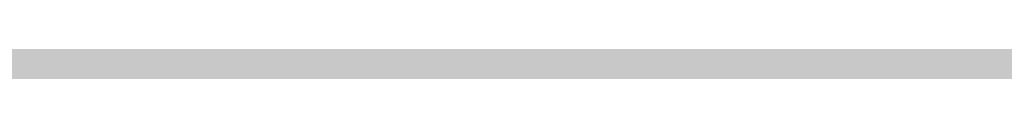
# Model space of a CAD drawing. Units: millimetres. Extents: x 0 to 2267, y 0 to 1823.
# Tile 205 of 256: x 1841.442 to 1842.748, y 1127.384 to 1127.404. Entities that reach past the tile are written whole.
import ezdxf

# ---------------------------------------------------------------- set-up
doc = ezdxf.new("R2010")
doc.units = ezdxf.units.MM
doc.header["$MEASUREMENT"] = 0
doc.layers.add('M-DIMS', color=2, linetype='Continuous', lineweight=25)
doc.layers.add('M-HATC', color=252, linetype='Continuous', lineweight=18)
doc.styles.get("Standard").update_dxf_attribs({"font": 'arial.ttf'})
doc.dimstyles.get("Standard").update_dxf_attribs({"dimtxt": 7, "dimasz": 4, "dimexe": 0.18, "dimexo": 0.0625, "dimgap": 0.09, "dimtad": 0, "dimdec": 0, "dimzin": 0, "dimdsep": 46, "dimtxsty": 'Standard', "dimcen": 0.09, "dimadec": 0, "dimazin": 0, "dimtfac": 1, "dimtdec": 0, "dimtofl": 0, "dimtmove": 0, "dimatfit": 3, "dimfxl": 1, "dimtolj": 1, "dimtzin": 0, "dimarcsym": 0})

# ---------------------------------------------------------------- blocks, each defined once
blk = doc.blocks.new('*D1')
at = {"layer": 'Defpoints', "color": 0, "transparency": 16777216}
for p in [(1593.4289, 1127.4171), (1843.4289, 1127.4171), (1843.4289, 955.6278)]:
    blk.add_point(p, dxfattribs=at)
at = {"layer": 'M-DIMS', "color": 0, "lineweight": -2, "transparency": 16777216}
for p, q in [((1593.4289, 1127.3546), (1593.4289, 955.4478)), ((1843.4289, 1127.3546), (1843.4289, 955.4478)), ((1597.4289, 955.6278), (1710.5582, 955.6278)), ((1839.4289, 955.6278), (1726.2996, 955.6278))]:
    blk.add_line(p, q, dxfattribs=at)
at = {"layer": 'M-DIMS', "color": 0, "transparency": 16777216}
for points in [[(1597.4289, 956.2944), (1597.4289, 954.9611), (1593.4289, 955.6278)], [(1839.4289, 956.2944), (1839.4289, 954.9611), (1843.4289, 955.6278)]]:
    blk.add_solid(points, dxfattribs=at)
at = {"layer": 'M-DIMS', "color": 0, "transparency": 16777216, "insert": (1718.4289, 955.6278), "char_height": 7, "attachment_point": 5}
blk.add_mtext('\\A1;250', dxfattribs=at)

msp = doc.modelspace()

# ---------------------------------------------------------------- hatches: boundary and pattern name
at = {"layer": 'M-HATC'}
h = msp.add_hatch(color=256, dxfattribs=at)
h.dxf.hatch_style = 1
h.paths.add_polyline_path([(2055.771, 1603.062), (1381.0868, 1603.062), (1381.0868, 1598.062), (2055.771, 1598.062)])
h.paths.add_polyline_path([(2055.771, 1598.062), (1381.0868, 1598.062), (1381.0868, 1593.062), (2055.771, 1593.062)])
h.paths.add_polyline_path([(2051.3074, 1536.7609), (1385.5504, 1536.7609), (1385.5504, 1526.7609), (1387.5504, 1526.7609), (1388.5366, 1525.0528), (1385.3319, 1521.2335), (1385.3319, 1521.2226), (2050.2542, 1522.7491), (2048.3212, 1525.0528), (2049.3074, 1526.7609), (2051.3074, 1526.7609)])
edge = h.paths.add_edge_path()
edge.add_arc((1847.5345, 1379.1492), 135, 222.603061, 222.890851, ccw=False)
edge.add_line((1748.1663, 1287.7656), (1683.0921, 1287.7656))
edge.add_arc((1583.7239, 1379.1492), 135, 317.109149, 317.396939, ccw=False)
edge.add_arc((1678.9686, 1290.6707), 5, 222.8909, 317.1091, ccw=False)
edge.add_arc((1774.2133, 1379.1492), 135, 222.603061, 222.890851, ccw=False)
edge.add_line((1674.8451, 1287.7656), (1609.7709, 1287.7656))
edge.add_arc((1510.4027, 1379.1492), 135, 317.109149, 317.396939, ccw=False)
edge.add_arc((1605.6474, 1290.6707), 5, 222.8909, 317.1091, ccw=False)
edge.add_arc((1700.8921, 1379.1492), 135, 222.603061, 222.890851, ccw=False)
edge.add_line((1601.5239, 1287.7656), (1536.4497, 1287.7656))
edge.add_arc((1437.0815, 1379.1492), 135, 317.109149, 317.396939, ccw=False)
edge.add_arc((1532.3262, 1290.6707), 5, 222.8909, 317.1091, ccw=False)
edge.add_arc((1627.5709, 1379.1492), 135, 222.603061, 222.890851, ccw=False)
edge.add_line((1528.2027, 1287.7656), (1505.9289, 1287.7656))
edge.add_spline(control_points=[(1505.9289, 1287.7656), (1504.2622, 1287.7656), (1504.2622, 1282.7656), (1505.9289, 1282.7656)], knot_values=[0, 0, 0, 0, 5, 5, 5, 5], degree=3, periodic=0)
edge.add_line((1505.9289, 1282.7656), (1930.9289, 1282.7656))
edge.add_spline(control_points=[(1930.9289, 1282.7656), (1932.5956, 1282.7656), (1932.5956, 1287.7656), (1930.9289, 1287.7656)], knot_values=[0, 0, 0, 0, 5, 5, 5, 5], degree=3, periodic=0)
edge.add_line((1930.9289, 1287.7656), (1903.0557, 1287.7656))
edge.add_arc((1803.6875, 1379.1492), 135, 317.109149, 317.396939, ccw=False)
edge.add_arc((1898.9322, 1290.6707), 5, 222.8909, 317.1091, ccw=False)
edge.add_arc((1994.1769, 1379.1492), 135, 222.603061, 222.890851, ccw=False)
edge.add_line((1894.8087, 1287.7656), (1829.7345, 1287.7656))
edge.add_arc((1730.3663, 1379.1492), 135, 317.109149, 317.396939, ccw=False)
edge.add_arc((1825.611, 1290.6707), 5, 222.8909, 317.1091, ccw=False)
edge.add_arc((1920.8557, 1379.1492), 135, 222.603061, 222.890851, ccw=False)
edge.add_line((1821.4875, 1287.7656), (1756.4133, 1287.7656))
edge.add_arc((1657.0451, 1379.1492), 135, 317.109149, 317.396939, ccw=False)
edge.add_arc((1752.2898, 1290.6707), 5, 222.8909, 317.1091, ccw=False)
edge = h.paths.add_edge_path()
edge.add_spline(control_points=[(1843.4289, 1227.2475), (1845.0956, 1227.2475), (1845.0956, 1232.2475), (1843.4289, 1232.2475)], knot_values=[0, 0, 0, 0, 5, 5, 5, 5], degree=3, periodic=0)
edge.add_line((1843.4289, 1232.2475), (1593.4289, 1232.2475))
edge.add_spline(control_points=[(1593.4289, 1232.2475), (1591.7622, 1232.2475), (1591.7622, 1227.2475), (1593.4289, 1227.2475)], knot_values=[0, 0, 0, 0, 5, 5, 5, 5], degree=3, periodic=0)
edge.add_line((1593.4289, 1227.2475), (1843.4289, 1227.2475))
h.paths.add_polyline_path([(1905.9289, 1127.4171), (1530.9289, 1127.4171, 0.414214), (1520.9289, 1117.4171), (1530.9289, 1117.4171), (1915.9289, 1117.4171, 0.414214)])
edge = h.paths.add_edge_path()
edge.add_arc((1397.0858, 1498.4078), 12.7299, 90.78215, 190.87871, ccw=False)
edge.add_line((1396.912, 1511.1365), (1428.0097, 1511.3488))
edge.add_line((1428.0097, 1511.3488), (1433.0097, 1511.3488))
edge.add_line((1433.0097, 1511.3488), (1434.439, 1511.3488))
edge.add_arc((1419.474, 1498.0804), 20, 41.561, 74.08211)
edge.add_line((1424.9592, 1517.3135), (1399.9351, 1517.2561))
edge.add_spline(control_points=[(1399.9307, 1517.2561), (1399.884, 1517.2131), (1399.8328, 1517.1689), (1399.7774, 1517.1236)], knot_values=[11.567499, 11.567499, 11.567499, 11.567499, 11.814249, 11.814249, 11.814249, 11.814249], degree=3, periodic=0)
edge.add_spline(control_points=[(1399.6328, 1517.0099), (1399.5831, 1516.9721), (1399.5307, 1516.9338), (1399.4759, 1516.8947)], knot_values=[11.167718, 11.167718, 11.167718, 11.167718, 11.365188, 11.365188, 11.365188, 11.365188], degree=3, periodic=0)
edge.add_spline(control_points=[(1399.3398, 1516.8001), (1399.1514, 1516.6719), (1398.9384, 1516.5377), (1398.704, 1516.3994)], knot_values=[10.376405, 10.376405, 10.376405, 10.376405, 11.00994, 11.00994, 11.00994, 11.00994], degree=3, periodic=0)
edge.add_spline(control_points=[(1398.6572, 1516.3719), (1398.5789, 1516.326), (1398.4983, 1516.2797), (1398.4155, 1516.2331)], knot_values=[10.125175, 10.125175, 10.125175, 10.125175, 10.334406, 10.334406, 10.334406, 10.334406], degree=3, periodic=0)
edge.add_spline(control_points=[(1398.2642, 1516.1487), (1398.196, 1516.1111), (1398.1263, 1516.0732), (1398.0555, 1516.0351)], knot_values=[9.832246, 9.832246, 9.832246, 9.832246, 9.999658, 9.999658, 9.999658, 9.999658], degree=3, periodic=0)
edge.add_spline(control_points=[(1397.9987, 1516.0048), (1397.7312, 1515.8621), (1397.446, 1515.7171), (1397.1466, 1515.5714)], knot_values=[9.161808, 9.161808, 9.161808, 9.161808, 9.787769, 9.787769, 9.787769, 9.787769], degree=3, periodic=0)
edge.add_spline(control_points=[(1397.1466, 1515.5714), (1396.8418, 1515.423), (1396.5222, 1515.274), (1396.1914, 1515.1262)], knot_values=[8.524455, 8.524455, 8.524455, 8.524455, 9.161808, 9.161808, 9.161808, 9.161808], degree=3, periodic=0)
edge.add_spline(control_points=[(1396.0777, 1515.0756), (1395.9854, 1515.0348), (1395.8922, 1514.994), (1395.7983, 1514.9534)], knot_values=[8.275193, 8.275193, 8.275193, 8.275193, 8.451726, 8.451726, 8.451726, 8.451726], degree=3, periodic=0)
edge.add_spline(control_points=[(1395.6018, 1514.8691), (1395.4997, 1514.8257), (1395.3968, 1514.7824), (1395.2932, 1514.7394)], knot_values=[7.962917, 7.962917, 7.962917, 7.962917, 8.152764, 8.152764, 8.152764, 8.152764], degree=3, periodic=0)
edge.add_spline(control_points=[(1395.2116, 1514.7057), (1394.8278, 1514.5475), (1394.4345, 1514.3929), (1394.0364, 1514.2442)], knot_values=[7.21254, 7.21254, 7.21254, 7.21254, 7.913148, 7.913148, 7.913148, 7.913148], degree=3, periodic=0)
edge.add_spline(control_points=[(1394.0364, 1514.2442), (1393.7076, 1514.1214), (1393.3754, 1514.0027), (1393.0427, 1513.8895)], knot_values=[6.633733, 6.633733, 6.633733, 6.633733, 7.21254, 7.21254, 7.21254, 7.21254], degree=3, periodic=0)
edge.add_spline(control_points=[(1392.8214, 1513.815), (1392.7198, 1513.7812), (1392.6181, 1513.7479), (1392.5166, 1513.7152)], knot_values=[6.328796, 6.328796, 6.328796, 6.328796, 6.505493, 6.505493, 6.505493, 6.505493], degree=3, periodic=0)
edge.add_spline(control_points=[(1392.5166, 1513.7152), (1392.3187, 1513.6515), (1392.1212, 1513.59), (1391.9244, 1513.531)], knot_values=[5.984605, 5.984605, 5.984605, 5.984605, 6.328796, 6.328796, 6.328796, 6.328796], degree=3, periodic=0)
edge.add_spline(control_points=[(1391.7915, 1513.4915), (1391.3122, 1513.3501), (1390.8384, 1513.2239), (1390.3784, 1513.1171)], knot_values=[5.066697, 5.066697, 5.066697, 5.066697, 5.907055, 5.907055, 5.907055, 5.907055], degree=3, periodic=0)
edge.add_spline(control_points=[(1390.3784, 1513.1171), (1390.1797, 1513.071), (1389.9836, 1513.0284), (1389.7907, 1512.9899)], knot_values=[4.70367, 4.70367, 4.70367, 4.70367, 5.066695, 5.066695, 5.066695, 5.066695], degree=3, periodic=0)
edge.add_spline(control_points=[(1389.422, 1512.9204), (1389.2459, 1512.8892), (1389.0729, 1512.8617), (1388.9036, 1512.8381)], knot_values=[4.130571, 4.130571, 4.130571, 4.130571, 4.469816, 4.469816, 4.469816, 4.469816], degree=3, periodic=0)
edge.add_spline(control_points=[(1388.9036, 1512.8381), (1388.591, 1512.7946), (1388.2911, 1512.7644), (1388.0071, 1512.7494)], knot_values=[3.504031, 3.504031, 3.504031, 3.504031, 4.130571, 4.130571, 4.130571, 4.130571], degree=3, periodic=0)
edge.add_spline(control_points=[(1387.9356, 1512.7459), (1387.8538, 1512.7423), (1387.7733, 1512.74), (1387.6944, 1512.739)], knot_values=[3.268866, 3.268866, 3.268866, 3.268866, 3.451164, 3.451164, 3.451164, 3.451164], degree=3, periodic=0)
edge.add_spline(control_points=[(1387.3351, 1512.7443), (1387.2076, 1512.7499), (1387.0847, 1512.7597), (1386.967, 1512.7739)], knot_values=[2.670686, 2.670686, 2.670686, 2.670686, 2.984, 2.984, 2.984, 2.984], degree=3, periodic=0)
edge.add_spline(control_points=[(1386.8327, 1512.7922), (1386.8209, 1512.7941), (1386.8092, 1512.7959), (1386.7975, 1512.7979)], knot_values=[2.516981, 2.516981, 2.516981, 2.516981, 2.549528, 2.549528, 2.549528, 2.549528], degree=3, periodic=0)
edge.add_spline(control_points=[(1386.4526, 1512.8735), (1386.4257, 1512.881), (1386.3993, 1512.889), (1386.3733, 1512.8972)], knot_values=[2.095869, 2.095869, 2.095869, 2.095869, 2.17941, 2.17941, 2.17941, 2.17941], degree=3, periodic=0)
edge.add_spline(control_points=[(1386.0691, 1513.0189), (1386.0634, 1513.0217), (1386.0577, 1513.0246), (1386.052, 1513.0275)], knot_values=[1.72453, 1.72453, 1.72453, 1.72453, 1.745933, 1.745933, 1.745933, 1.745933], degree=3, periodic=0)
edge.add_arc((1399.474, 1498.0804), 20, 131.82432, 180)
edge.add_arc((1630.3336, 1505.5484), 250.9708, 181.705176, 236.427975)
edge.add_arc((1605.3399, 1483.3044), 218.7822, 238.660829, 243.34961)
edge.add_arc((1647.0911, 1510.3592), 262.8986, 183.129836, 237.853442, ccw=False)
h.paths.add_polyline_path([(1406.5369, 1391.9644, 0.149382), (1491.5506, 1296.4418, -0.129517)], flags=17)
edge = h.paths.add_edge_path()
edge.add_arc((2037.3838, 1498.0804), 20, 0, 48.26587)
edge.add_spline(control_points=[(2050.6973, 1513.0052), (2050.6512, 1512.9847), (2050.6034, 1512.9655), (2050.5539, 1512.9477)], knot_values=[1.835652, 1.835652, 1.835652, 1.835652, 2.000781, 2.000781, 2.000781, 2.000781], degree=3, periodic=0)
edge.add_spline(control_points=[(2050.4616, 1512.9166), (2050.479, 1512.9221), (2050.4963, 1512.9277), (2050.5133, 1512.9335)], knot_values=[2.045477, 2.045477, 2.045477, 2.045477, 2.101389, 2.101389, 2.101389, 2.101389], degree=3, periodic=0)
edge.add_spline(control_points=[(2050.129, 1512.8342), (2050.1984, 1512.8473), (2050.2657, 1512.8623), (2050.3308, 1512.8792)], knot_values=[2.237629, 2.237629, 2.237629, 2.237629, 2.435841, 2.435841, 2.435841, 2.435841], degree=3, periodic=0)
edge.add_spline(control_points=[(2050.0946, 1512.8278), (2050.1061, 1512.8299), (2050.1176, 1512.832), (2050.129, 1512.8342)], knot_values=[2.435841, 2.435841, 2.435841, 2.435841, 2.468321, 2.468321, 2.468321, 2.468321], degree=3, periodic=0)
edge.add_spline(control_points=[(2049.7843, 1512.7851), (2049.8552, 1512.7922), (2049.9243, 1512.8008), (2049.9917, 1512.8109)], knot_values=[2.563852, 2.563852, 2.563852, 2.563852, 2.748541, 2.748541, 2.748541, 2.748541], degree=3, periodic=0)
edge.add_spline(control_points=[(2049.4052, 1512.7617), (2049.5364, 1512.7653), (2049.6629, 1512.773), (2049.7843, 1512.7851)], knot_values=[2.748541, 2.748541, 2.748541, 2.748541, 3.064882, 3.064882, 3.064882, 3.064882], degree=3, periodic=0)
edge.add_spline(control_points=[(2049.1698, 1512.7597), (2049.2336, 1512.7591), (2049.2965, 1512.7594), (2049.3584, 1512.7606)], knot_values=[3.102309, 3.102309, 3.102309, 3.102309, 3.2503, 3.2503, 3.2503, 3.2503], degree=3, periodic=0)
edge.add_spline(control_points=[(2048.8573, 1512.7691), (2048.9638, 1512.7638), (2049.068, 1512.7606), (2049.1698, 1512.7597)], knot_values=[3.2503, 3.2503, 3.2503, 3.2503, 3.486069, 3.486069, 3.486069, 3.486069], degree=3, periodic=0)
edge.add_spline(control_points=[(2048.6924, 1512.7789), (2048.3729, 1512.8009), (2048.0345, 1512.8411), (2047.6817, 1512.897)], knot_values=[3.606429, 3.606429, 3.606429, 3.606429, 4.2989, 4.2989, 4.2989, 4.2989], degree=3, periodic=0)
edge.add_spline(control_points=[(2047.6817, 1512.897), (2047.5458, 1512.9185), (2047.4077, 1512.9424), (2047.2678, 1512.9685)], knot_values=[4.2989, 4.2989, 4.2989, 4.2989, 4.565769, 4.565769, 4.565769, 4.565769], degree=3, periodic=0)
edge.add_spline(control_points=[(2047.2678, 1512.9685), (2047.1449, 1512.9914), (2047.0207, 1513.016), (2046.8951, 1513.0422)], knot_values=[4.565769, 4.565769, 4.565769, 4.565769, 4.799971, 4.799971, 4.799971, 4.799971], degree=3, periodic=0)
edge.add_spline(control_points=[(2046.8951, 1513.0422), (2046.5286, 1513.1188), (2046.1513, 1513.209), (2045.7676, 1513.3107)], knot_values=[4.799971, 4.799971, 4.799971, 4.799971, 5.483718, 5.483718, 5.483718, 5.483718], degree=3, periodic=0)
edge.add_spline(control_points=[(2045.7676, 1513.3107), (2045.3724, 1513.4154), (2044.9704, 1513.5322), (2044.5662, 1513.6588)], knot_values=[5.483718, 5.483718, 5.483718, 5.483718, 6.187866, 6.187866, 6.187866, 6.187866], degree=3, periodic=0)
edge.add_spline(control_points=[(2044.5662, 1513.6588), (2044.4149, 1513.7061), (2044.2633, 1513.7549), (2044.1116, 1513.8048)], knot_values=[6.187866, 6.187866, 6.187866, 6.187866, 6.451551, 6.451551, 6.451551, 6.451551], degree=3, periodic=0)
edge.add_spline(control_points=[(2044.1116, 1513.8048), (2043.9967, 1513.8427), (2043.8817, 1513.8813), (2043.7668, 1513.9205)], knot_values=[6.451551, 6.451551, 6.451551, 6.451551, 6.651434, 6.651434, 6.651434, 6.651434], degree=3, periodic=0)
edge.add_spline(control_points=[(2043.7668, 1513.9205), (2043.3716, 1514.0554), (2042.9774, 1514.1979), (2042.5886, 1514.3458)], knot_values=[6.651434, 6.651434, 6.651434, 6.651434, 7.338879, 7.338879, 7.338879, 7.338879], degree=3, periodic=0)
edge.add_spline(control_points=[(2042.5886, 1514.3458), (2042.1643, 1514.5071), (2041.7465, 1514.6749), (2041.3409, 1514.846)], knot_values=[7.338879, 7.338879, 7.338879, 7.338879, 8.089209, 8.089209, 8.089209, 8.089209], degree=3, periodic=0)
edge.add_spline(control_points=[(2041.3409, 1514.846), (2041.1028, 1514.9465), (2040.869, 1515.0481), (2040.6405, 1515.1502)], knot_values=[8.089209, 8.089209, 8.089209, 8.089209, 8.529587, 8.529587, 8.529587, 8.529587], degree=3, periodic=0)
edge.add_spline(control_points=[(2040.51, 1515.2089), (2040.0824, 1515.4022), (2039.6747, 1515.5971), (2039.295, 1515.7894)], knot_values=[8.613818, 8.613818, 8.613818, 8.613818, 9.44571, 9.44571, 9.44571, 9.44571], degree=3, periodic=0)
edge.add_spline(control_points=[(2039.295, 1515.7894), (2039.0618, 1515.9075), (2038.8391, 1516.0246), (2038.6288, 1516.1398)], knot_values=[9.44571, 9.44571, 9.44571, 9.44571, 9.956404, 9.956404, 9.956404, 9.956404], degree=3, periodic=0)
edge.add_spline(control_points=[(2038.6288, 1516.1398), (2038.5187, 1516.2001), (2038.4121, 1516.2598), (2038.309, 1516.3189)], knot_values=[9.956404, 9.956404, 9.956404, 9.956404, 10.223542, 10.223542, 10.223542, 10.223542], degree=3, periodic=0)
edge.add_spline(control_points=[(2038.309, 1516.3189), (2038.2138, 1516.3735), (2038.1216, 1516.4276), (2038.0328, 1516.481)], knot_values=[10.223542, 10.223542, 10.223542, 10.223542, 10.47051, 10.47051, 10.47051, 10.47051], degree=3, periodic=0)
edge.add_spline(control_points=[(2038.0328, 1516.481), (2037.7855, 1516.6296), (2037.5639, 1516.773), (2037.3722, 1516.909)], knot_values=[10.47051, 10.47051, 10.47051, 10.47051, 11.15767, 11.15767, 11.15767, 11.15767], degree=3, periodic=0)
edge.add_spline(control_points=[(2037.3722, 1516.909), (2037.2789, 1516.9752), (2037.1927, 1517.0396), (2037.1142, 1517.102)], knot_values=[11.15767, 11.15767, 11.15767, 11.15767, 11.49227, 11.49227, 11.49227, 11.49227], degree=3, periodic=0)
edge.add_spline(control_points=[(2036.8564, 1517.3259), (2036.9148, 1517.2692), (2036.9814, 1517.2103), (2037.0557, 1517.1492)], knot_values=[11.577341, 11.577341, 11.577341, 11.577341, 11.91035, 11.91035, 11.91035, 11.91035], degree=3, periodic=0)
edge.add_spline(control_points=[(2036.8074, 1517.3748), (2036.823, 1517.3587), (2036.8393, 1517.3424), (2036.8564, 1517.3259)], knot_values=[11.91035, 11.91035, 11.91035, 11.91035, 12.007402, 12.007402, 12.007402, 12.007402], degree=3, periodic=0)
edge.add_spline(control_points=[(2036.7017, 1517.494), (2036.7104, 1517.483), (2036.7196, 1517.4719), (2036.7291, 1517.4606)], knot_values=[12.184155, 12.184155, 12.184155, 12.184155, 12.255409, 12.255409, 12.255409, 12.255409], degree=3, periodic=0)
edge.add_spline(control_points=[(2036.6159, 1517.6205), (2036.62, 1517.613), (2036.6243, 1517.6055), (2036.6289, 1517.5979)], knot_values=[12.487913, 12.487913, 12.487913, 12.487913, 12.541035, 12.541035, 12.541035, 12.541035], degree=3, periodic=0)
edge.add_spline(control_points=[(2036.5635, 1517.786), (2036.5637, 1517.7794), (2036.5642, 1517.7726), (2036.565, 1517.7658)], knot_values=[12.911761, 12.911761, 12.911761, 12.911761, 12.968286, 12.968286, 12.968286, 12.968286], degree=3, periodic=0)
edge.add_spline(control_points=[(2036.6166, 1517.9304), (2036.6125, 1517.9259), (2036.6086, 1517.9212), (2036.6049, 1517.9165)], knot_values=[13.382527, 13.382527, 13.382527, 13.382527, 13.433791, 13.433791, 13.433791, 13.433791], degree=3, periodic=0)
edge.add_spline(control_points=[(2036.749, 1518.017), (2036.7361, 1518.0116), (2036.7239, 1518.006), (2036.7124, 1518.0002)], knot_values=[13.726299, 13.726299, 13.726299, 13.726299, 13.809928, 13.809928, 13.809928, 13.809928], degree=3, periodic=0)
edge.add_spline(control_points=[(2036.8604, 1518.0528), (2036.8386, 1518.0474), (2036.8181, 1518.0416), (2036.7988, 1518.0353)], knot_values=[13.910887, 13.910887, 13.910887, 13.910887, 14.02153, 14.02153, 14.02153, 14.02153], degree=3, periodic=0)
edge.add_line((2036.9639, 1518.0804), (2032.3838, 1518.0804))
edge.add_line((2032.3838, 1518.0804), (2027.3838, 1518.0804))
edge.add_line((2027.3838, 1518.0804), (2022.3838, 1518.0804))
edge.add_line((2022.3838, 1518.0804), (2017.3838, 1518.0804))
edge.add_arc((2017.3838, 1498.0804), 20, 90, 138.439)
edge.add_line((2002.4188, 1511.3488), (2003.8481, 1511.3488))
edge.add_line((2003.8481, 1511.3488), (2008.8481, 1511.3488))
edge.add_line((2008.8481, 1511.3488), (2039.772, 1511.1377))
edge.add_arc((2039.772, 1498.4078), 12.7299, -10.87871, 90, ccw=False)
edge.add_arc((1789.7668, 1510.3592), 262.8986, 302.146558, 356.870164, ccw=False)
edge.add_arc((1831.5179, 1483.3044), 218.7822, 296.65039, 301.339171)
edge.add_arc((1806.5242, 1505.5484), 250.9708, 303.572025, 358.294824)
h.paths.add_polyline_path([(2030.321, 1391.9644, -0.129517), (1945.3072, 1296.4418, 0.149382)], flags=17)
edge = h.paths.add_edge_path()
edge.add_spline(control_points=[(2037.2464, 1518.0821), (2037.2898, 1518.081), (2037.3355, 1518.0804), (2037.3838, 1518.0804)], knot_values=[0.000012, 0.000012, 0.000012, 0.000012, 0.144754, 0.144754, 0.144754, 0.144754], degree=3, periodic=0)
edge.add_line((2037.3357, 1518.0804), (2037.0096, 1518.0804))
edge.add_spline(control_points=[(2037.0096, 1518.0804), (2036.9822, 1518.0768), (2036.956, 1518.0727), (2036.9312, 1518.0681)], knot_values=[14.13465, 14.13465, 14.13465, 14.13465, 14.247197, 14.247197, 14.247197, 14.247197], degree=3, periodic=0)
edge.add_spline(control_points=[(2036.9312, 1518.0681), (2036.9276, 1518.0674), (2036.9241, 1518.0667), (2036.9205, 1518.0661)], knot_values=[14.118315, 14.118315, 14.118315, 14.118315, 14.13465, 14.13465, 14.13465, 14.13465], degree=3, periodic=0)
edge.add_spline(control_points=[(2036.9205, 1518.0661), (2036.9118, 1518.0644), (2036.9032, 1518.0626), (2036.8948, 1518.0608)], knot_values=[14.078086, 14.078086, 14.078086, 14.078086, 14.118315, 14.118315, 14.118315, 14.118315], degree=3, periodic=0)
edge.add_spline(control_points=[(2036.8948, 1518.0608), (2036.883, 1518.0583), (2036.8716, 1518.0556), (2036.8604, 1518.0528)], knot_values=[14.02153, 14.02153, 14.02153, 14.02153, 14.078086, 14.078086, 14.078086, 14.078086], degree=3, periodic=0)
edge.add_spline(control_points=[(2036.8604, 1518.0528), (2036.8386, 1518.0474), (2036.8181, 1518.0416), (2036.7988, 1518.0353)], knot_values=[13.910887, 13.910887, 13.910887, 13.910887, 14.02153, 14.02153, 14.02153, 14.02153], degree=3, periodic=0)
edge.add_spline(control_points=[(2036.7988, 1518.0353), (2036.7981, 1518.035), (2036.7974, 1518.0348), (2036.7967, 1518.0346)], knot_values=[13.906906, 13.906906, 13.906906, 13.906906, 13.910887, 13.910887, 13.910887, 13.910887], degree=3, periodic=0)
edge.add_spline(control_points=[(2036.7967, 1518.0346), (2036.7882, 1518.0318), (2036.7799, 1518.0289), (2036.7719, 1518.0259)], knot_values=[13.857826, 13.857826, 13.857826, 13.857826, 13.906906, 13.906906, 13.906906, 13.906906], degree=3, periodic=0)
edge.add_spline(control_points=[(2036.7719, 1518.0259), (2036.764, 1518.023), (2036.7564, 1518.02), (2036.749, 1518.017)], knot_values=[13.809928, 13.809928, 13.809928, 13.809928, 13.857826, 13.857826, 13.857826, 13.857826], degree=3, periodic=0)
edge.add_spline(control_points=[(2036.749, 1518.017), (2036.7361, 1518.0116), (2036.7239, 1518.006), (2036.7124, 1518.0002)], knot_values=[13.726299, 13.726299, 13.726299, 13.726299, 13.809928, 13.809928, 13.809928, 13.809928], degree=3, periodic=0)
edge.add_spline(control_points=[(2036.7124, 1518.0002), (2036.7121, 1518), (2036.7118, 1517.9999), (2036.7115, 1517.9997)], knot_values=[13.723993, 13.723993, 13.723993, 13.723993, 13.726299, 13.726299, 13.726299, 13.726299], degree=3, periodic=0)
edge.add_spline(control_points=[(2036.7115, 1517.9997), (2036.7063, 1517.9971), (2036.7013, 1517.9944), (2036.6965, 1517.9917)], knot_values=[13.686536, 13.686536, 13.686536, 13.686536, 13.723993, 13.723993, 13.723993, 13.723993], degree=3, periodic=0)
edge.add_spline(control_points=[(2036.6965, 1517.9917), (2036.6919, 1517.9891), (2036.6874, 1517.9865), (2036.6831, 1517.9839)], knot_values=[13.651251, 13.651251, 13.651251, 13.651251, 13.686536, 13.686536, 13.686536, 13.686536], degree=3, periodic=0)
edge.add_spline(control_points=[(2036.6831, 1517.9839), (2036.6764, 1517.9798), (2036.67, 1517.9757), (2036.6639, 1517.9714)], knot_values=[13.596804, 13.596804, 13.596804, 13.596804, 13.651251, 13.651251, 13.651251, 13.651251], degree=3, periodic=0)
edge.add_spline(control_points=[(2036.6639, 1517.9714), (2036.6636, 1517.9712), (2036.6633, 1517.9709), (2036.6629, 1517.9707)], knot_values=[13.593956, 13.593956, 13.593956, 13.593956, 13.596804, 13.596804, 13.596804, 13.596804], degree=3, periodic=0)
edge.add_spline(control_points=[(2036.6629, 1517.9707), (2036.6603, 1517.9689), (2036.6577, 1517.967), (2036.6552, 1517.9651)], knot_values=[13.570322, 13.570322, 13.570322, 13.570322, 13.593956, 13.593956, 13.593956, 13.593956], degree=3, periodic=0)
edge.add_spline(control_points=[(2036.6552, 1517.9651), (2036.6525, 1517.9631), (2036.6499, 1517.9611), (2036.6474, 1517.9591)], knot_values=[13.545477, 13.545477, 13.545477, 13.545477, 13.570322, 13.570322, 13.570322, 13.570322], degree=3, periodic=0)
edge.add_spline(control_points=[(2036.6474, 1517.9591), (2036.6472, 1517.9589), (2036.6471, 1517.9588), (2036.6469, 1517.9587)], knot_values=[13.543931, 13.543931, 13.543931, 13.543931, 13.545477, 13.545477, 13.545477, 13.545477], degree=3, periodic=0)
edge.add_spline(control_points=[(2036.6469, 1517.9587), (2036.6412, 1517.9541), (2036.6358, 1517.9494), (2036.6307, 1517.9447)], knot_values=[13.488237, 13.488237, 13.488237, 13.488237, 13.543931, 13.543931, 13.543931, 13.543931], degree=3, periodic=0)
edge.add_spline(control_points=[(2036.6307, 1517.9447), (2036.6282, 1517.9423), (2036.6257, 1517.9399), (2036.6233, 1517.9374)], knot_values=[13.460307, 13.460307, 13.460307, 13.460307, 13.488237, 13.488237, 13.488237, 13.488237], degree=3, periodic=0)
edge.add_spline(control_points=[(2036.6233, 1517.9374), (2036.6215, 1517.9356), (2036.6198, 1517.9338), (2036.6181, 1517.932)], knot_values=[13.439712, 13.439712, 13.439712, 13.439712, 13.460307, 13.460307, 13.460307, 13.460307], degree=3, periodic=0)
edge.add_spline(control_points=[(2036.6181, 1517.932), (2036.6176, 1517.9315), (2036.6171, 1517.9309), (2036.6166, 1517.9304)], knot_values=[13.433791, 13.433791, 13.433791, 13.433791, 13.439712, 13.439712, 13.439712, 13.439712], degree=3, periodic=0)
edge.add_spline(control_points=[(2036.6166, 1517.9304), (2036.6125, 1517.9259), (2036.6086, 1517.9212), (2036.6049, 1517.9165)], knot_values=[13.382527, 13.382527, 13.382527, 13.382527, 13.433791, 13.433791, 13.433791, 13.433791], degree=3, periodic=0)
edge.add_spline(control_points=[(2036.6049, 1517.9165), (2036.6026, 1517.9135), (2036.6004, 1517.9104), (2036.5982, 1517.9074)], knot_values=[13.350017, 13.350017, 13.350017, 13.350017, 13.382527, 13.382527, 13.382527, 13.382527], degree=3, periodic=0)
edge.add_spline(control_points=[(2036.5982, 1517.9074), (2036.5972, 1517.9059), (2036.5962, 1517.9043), (2036.5952, 1517.9028)], knot_values=[13.333922, 13.333922, 13.333922, 13.333922, 13.350017, 13.350017, 13.350017, 13.350017], degree=3, periodic=0)
edge.add_spline(control_points=[(2036.5952, 1517.9028), (2036.5945, 1517.9018), (2036.5939, 1517.9009), (2036.5933, 1517.8999)], knot_values=[13.323828, 13.323828, 13.323828, 13.323828, 13.333922, 13.333922, 13.333922, 13.333922], degree=3, periodic=0)
edge.add_spline(control_points=[(2036.5933, 1517.8999), (2036.5905, 1517.8955), (2036.5879, 1517.8909), (2036.5855, 1517.8864)], knot_values=[13.277545, 13.277545, 13.277545, 13.277545, 13.323828, 13.323828, 13.323828, 13.323828], degree=3, periodic=0)
edge.add_spline(control_points=[(2036.5855, 1517.8864), (2036.5836, 1517.8827), (2036.5817, 1517.8789), (2036.5801, 1517.8751)], knot_values=[13.240119, 13.240119, 13.240119, 13.240119, 13.277545, 13.277545, 13.277545, 13.277545], degree=3, periodic=0)
edge.add_spline(control_points=[(2036.5801, 1517.8751), (2036.5795, 1517.8739), (2036.579, 1517.8727), (2036.5785, 1517.8715)], knot_values=[13.228211, 13.228211, 13.228211, 13.228211, 13.240119, 13.240119, 13.240119, 13.240119], degree=3, periodic=0)
edge.add_spline(control_points=[(2036.5785, 1517.8715), (2036.578, 1517.8702), (2036.5774, 1517.869), (2036.5769, 1517.8677)], knot_values=[13.215717, 13.215717, 13.215717, 13.215717, 13.228211, 13.228211, 13.228211, 13.228211], degree=3, periodic=0)
edge.add_spline(control_points=[(2036.5769, 1517.8677), (2036.5755, 1517.864), (2036.5741, 1517.8603), (2036.5729, 1517.8565)], knot_values=[13.179847, 13.179847, 13.179847, 13.179847, 13.215717, 13.215717, 13.215717, 13.215717], degree=3, periodic=0)
edge.add_spline(control_points=[(2036.5729, 1517.8565), (2036.5713, 1517.8515), (2036.5699, 1517.8464), (2036.5687, 1517.8413)], knot_values=[13.132017, 13.132017, 13.132017, 13.132017, 13.179847, 13.179847, 13.179847, 13.179847], degree=3, periodic=0)
edge.add_spline(control_points=[(2036.5687, 1517.8413), (2036.5684, 1517.8402), (2036.5682, 1517.8392), (2036.568, 1517.8382)], knot_values=[13.122482, 13.122482, 13.122482, 13.122482, 13.132017, 13.132017, 13.132017, 13.132017], degree=3, periodic=0)
edge.add_spline(control_points=[(2036.568, 1517.8382), (2036.5676, 1517.8363), (2036.5672, 1517.8345), (2036.5669, 1517.8327)], knot_values=[13.105592, 13.105592, 13.105592, 13.105592, 13.122482, 13.122482, 13.122482, 13.122482], degree=3, periodic=0)
edge.add_spline(control_points=[(2036.5669, 1517.8327), (2036.5662, 1517.8292), (2036.5657, 1517.8257), (2036.5652, 1517.8222)], knot_values=[13.074063, 13.074063, 13.074063, 13.074063, 13.105592, 13.105592, 13.105592, 13.105592], degree=3, periodic=0)
edge.add_spline(control_points=[(2036.5652, 1517.8222), (2036.5652, 1517.8222), (2036.5652, 1517.8222), (2036.5652, 1517.8222)], knot_values=[13.074043, 13.074043, 13.074043, 13.074043, 13.074063, 13.074063, 13.074063, 13.074063], degree=3, periodic=0)
edge.add_spline(control_points=[(2036.5652, 1517.8222), (2036.5644, 1517.8164), (2036.5639, 1517.8106), (2036.5636, 1517.8046)], knot_values=[13.021884, 13.021884, 13.021884, 13.021884, 13.074043, 13.074043, 13.074043, 13.074043], degree=3, periodic=0)
edge.add_spline(control_points=[(2036.5636, 1517.8046), (2036.5636, 1517.804), (2036.5636, 1517.8034), (2036.5635, 1517.8028)], knot_values=[13.01674, 13.01674, 13.01674, 13.01674, 13.021884, 13.021884, 13.021884, 13.021884], degree=3, periodic=0)
edge.add_spline(control_points=[(2036.5635, 1517.8028), (2036.5634, 1517.8005), (2036.5634, 1517.7982), (2036.5634, 1517.7958)], knot_values=[12.996438, 12.996438, 12.996438, 12.996438, 13.01674, 13.01674, 13.01674, 13.01674], degree=3, periodic=0)
edge.add_spline(control_points=[(2036.5634, 1517.7958), (2036.5633, 1517.7926), (2036.5634, 1517.7893), (2036.5635, 1517.786)], knot_values=[12.968286, 12.968286, 12.968286, 12.968286, 12.996438, 12.996438, 12.996438, 12.996438], degree=3, periodic=0)
edge.add_spline(control_points=[(2036.5635, 1517.786), (2036.5637, 1517.7794), (2036.5642, 1517.7726), (2036.565, 1517.7658)], knot_values=[12.911761, 12.911761, 12.911761, 12.911761, 12.968286, 12.968286, 12.968286, 12.968286], degree=3, periodic=0)
edge.add_spline(control_points=[(2036.565, 1517.7658), (2036.565, 1517.7657), (2036.565, 1517.7656), (2036.565, 1517.7656)], knot_values=[12.911017, 12.911017, 12.911017, 12.911017, 12.911761, 12.911761, 12.911761, 12.911761], degree=3, periodic=0)
edge.add_spline(control_points=[(2036.565, 1517.7656), (2036.5654, 1517.7625), (2036.5658, 1517.7593), (2036.5663, 1517.7562)], knot_values=[12.88528, 12.88528, 12.88528, 12.88528, 12.911017, 12.911017, 12.911017, 12.911017], degree=3, periodic=0)
edge.add_spline(control_points=[(2036.5663, 1517.7562), (2036.5667, 1517.7534), (2036.5672, 1517.7506), (2036.5677, 1517.7478)], knot_values=[12.862519, 12.862519, 12.862519, 12.862519, 12.88528, 12.88528, 12.88528, 12.88528], degree=3, periodic=0)
edge.add_spline(control_points=[(2036.5677, 1517.7478), (2036.5678, 1517.7474), (2036.5679, 1517.7469), (2036.568, 1517.7465)], knot_values=[12.858885, 12.858885, 12.858885, 12.858885, 12.862519, 12.862519, 12.862519, 12.862519], degree=3, periodic=0)
edge.add_spline(control_points=[(2036.568, 1517.7465), (2036.5692, 1517.7399), (2036.5707, 1517.7332), (2036.5724, 1517.7264)], knot_values=[12.8053, 12.8053, 12.8053, 12.8053, 12.858885, 12.858885, 12.858885, 12.858885], degree=3, periodic=0)
edge.add_spline(control_points=[(2036.5724, 1517.7264), (2036.5734, 1517.7226), (2036.5745, 1517.7187), (2036.5756, 1517.7149)], knot_values=[12.775176, 12.775176, 12.775176, 12.775176, 12.8053, 12.8053, 12.8053, 12.8053], degree=3, periodic=0)
edge.add_spline(control_points=[(2036.5756, 1517.7149), (2036.5763, 1517.7125), (2036.577, 1517.7102), (2036.5778, 1517.7078)], knot_values=[12.756759, 12.756759, 12.756759, 12.756759, 12.775176, 12.775176, 12.775176, 12.775176], degree=3, periodic=0)
edge.add_spline(control_points=[(2036.5778, 1517.7078), (2036.5781, 1517.7067), (2036.5784, 1517.7057), (2036.5787, 1517.7047)], knot_values=[12.748742, 12.748742, 12.748742, 12.748742, 12.756759, 12.756759, 12.756759, 12.756759], degree=3, periodic=0)
edge.add_spline(control_points=[(2036.5787, 1517.7047), (2036.5808, 1517.6983), (2036.5831, 1517.6919), (2036.5856, 1517.6854)], knot_values=[12.69959, 12.69959, 12.69959, 12.69959, 12.748742, 12.748742, 12.748742, 12.748742], degree=3, periodic=0)
edge.add_spline(control_points=[(2036.5856, 1517.6854), (2036.5876, 1517.68), (2036.5898, 1517.6746), (2036.5921, 1517.6692)], knot_values=[12.659038, 12.659038, 12.659038, 12.659038, 12.69959, 12.69959, 12.69959, 12.69959], degree=3, periodic=0)
edge.add_spline(control_points=[(2036.5921, 1517.6692), (2036.594, 1517.6648), (2036.5959, 1517.6605), (2036.5979, 1517.6561)], knot_values=[12.626806, 12.626806, 12.626806, 12.626806, 12.659038, 12.659038, 12.659038, 12.659038], degree=3, periodic=0)
edge.add_spline(control_points=[(2036.5979, 1517.6561), (2036.5984, 1517.6551), (2036.5989, 1517.6541), (2036.5993, 1517.6531)], knot_values=[12.619394, 12.619394, 12.619394, 12.619394, 12.626806, 12.626806, 12.626806, 12.626806], degree=3, periodic=0)
edge.add_spline(control_points=[(2036.5993, 1517.6531), (2036.6043, 1517.6424), (2036.6099, 1517.6315), (2036.6159, 1517.6205)], knot_values=[12.541039, 12.541039, 12.541039, 12.541039, 12.619394, 12.619394, 12.619394, 12.619394], degree=3, periodic=0)
edge.add_spline(control_points=[(2036.6159, 1517.6205), (2036.6159, 1517.6205), (2036.6159, 1517.6205), (2036.6159, 1517.6205)], knot_values=[12.541035, 12.541035, 12.541035, 12.541035, 12.541039, 12.541039, 12.541039, 12.541039], degree=3, periodic=0)
edge.add_spline(control_points=[(2036.6159, 1517.6205), (2036.62, 1517.613), (2036.6243, 1517.6055), (2036.6289, 1517.5979)], knot_values=[12.487913, 12.487913, 12.487913, 12.487913, 12.541035, 12.541035, 12.541035, 12.541035], degree=3, periodic=0)
edge.add_spline(control_points=[(2036.6289, 1517.5979), (2036.6326, 1517.5916), (2036.6365, 1517.5853), (2036.6406, 1517.5789)], knot_values=[12.443982, 12.443982, 12.443982, 12.443982, 12.487913, 12.487913, 12.487913, 12.487913], degree=3, periodic=0)
edge.add_spline(control_points=[(2036.6406, 1517.5789), (2036.6414, 1517.5776), (2036.6423, 1517.5763), (2036.6431, 1517.5749)], knot_values=[12.434996, 12.434996, 12.434996, 12.434996, 12.443982, 12.443982, 12.443982, 12.443982], degree=3, periodic=0)
edge.add_spline(control_points=[(2036.6431, 1517.5749), (2036.6531, 1517.5596), (2036.6639, 1517.5439), (2036.6756, 1517.528)], knot_values=[12.329647, 12.329647, 12.329647, 12.329647, 12.434996, 12.434996, 12.434996, 12.434996], degree=3, periodic=0)
edge.add_spline(control_points=[(2036.6756, 1517.528), (2036.6839, 1517.5168), (2036.6925, 1517.5055), (2036.7017, 1517.494)], knot_values=[12.255409, 12.255409, 12.255409, 12.255409, 12.329647, 12.329647, 12.329647, 12.329647], degree=3, periodic=0)
edge.add_spline(control_points=[(2036.7017, 1517.494), (2036.7104, 1517.483), (2036.7196, 1517.4719), (2036.7291, 1517.4606)], knot_values=[12.184155, 12.184155, 12.184155, 12.184155, 12.255409, 12.255409, 12.255409, 12.255409], degree=3, periodic=0)
edge.add_spline(control_points=[(2036.7291, 1517.4606), (2036.7436, 1517.4435), (2036.759, 1517.4262), (2036.7753, 1517.4085)], knot_values=[12.075961, 12.075961, 12.075961, 12.075961, 12.184155, 12.184155, 12.184155, 12.184155], degree=3, periodic=0)
edge.add_spline(control_points=[(2036.7753, 1517.4085), (2036.7763, 1517.4075), (2036.7773, 1517.4064), (2036.7783, 1517.4054)], knot_values=[12.069502, 12.069502, 12.069502, 12.069502, 12.075961, 12.075961, 12.075961, 12.075961], degree=3, periodic=0)
edge.add_spline(control_points=[(2036.7783, 1517.4054), (2036.7877, 1517.3953), (2036.7974, 1517.385), (2036.8074, 1517.3748)], knot_values=[12.007402, 12.007402, 12.007402, 12.007402, 12.069502, 12.069502, 12.069502, 12.069502], degree=3, periodic=0)
edge.add_spline(control_points=[(2036.8074, 1517.3748), (2036.823, 1517.3587), (2036.8393, 1517.3424), (2036.8564, 1517.3259)], knot_values=[11.91035, 11.91035, 11.91035, 11.91035, 12.007402, 12.007402, 12.007402, 12.007402], degree=3, periodic=0)
edge.add_spline(control_points=[(2036.8564, 1517.3259), (2036.9148, 1517.2692), (2036.9814, 1517.2103), (2037.0557, 1517.1492)], knot_values=[11.577341, 11.577341, 11.577341, 11.577341, 11.91035, 11.91035, 11.91035, 11.91035], degree=3, periodic=0)
edge.add_spline(control_points=[(2037.0557, 1517.1492), (2037.0747, 1517.1336), (2037.0942, 1517.1179), (2037.1142, 1517.102)], knot_values=[11.49227, 11.49227, 11.49227, 11.49227, 11.577341, 11.577341, 11.577341, 11.577341], degree=3, periodic=0)
edge.add_spline(control_points=[(2037.1142, 1517.102), (2037.1927, 1517.0396), (2037.2789, 1516.9752), (2037.3722, 1516.909)], knot_values=[11.15767, 11.15767, 11.15767, 11.15767, 11.49227, 11.49227, 11.49227, 11.49227], degree=3, periodic=0)
edge.add_spline(control_points=[(2037.3722, 1516.909), (2037.5639, 1516.773), (2037.7855, 1516.6296), (2038.0328, 1516.481)], knot_values=[10.47051, 10.47051, 10.47051, 10.47051, 11.15767, 11.15767, 11.15767, 11.15767], degree=3, periodic=0)
edge.add_spline(control_points=[(2038.0328, 1516.481), (2038.1216, 1516.4276), (2038.2138, 1516.3735), (2038.309, 1516.3189)], knot_values=[10.223542, 10.223542, 10.223542, 10.223542, 10.47051, 10.47051, 10.47051, 10.47051], degree=3, periodic=0)
edge.add_spline(control_points=[(2038.309, 1516.3189), (2038.4121, 1516.2598), (2038.5187, 1516.2001), (2038.6288, 1516.1398)], knot_values=[9.956404, 9.956404, 9.956404, 9.956404, 10.223542, 10.223542, 10.223542, 10.223542], degree=3, periodic=0)
edge.add_spline(control_points=[(2038.6288, 1516.1398), (2038.8391, 1516.0246), (2039.0618, 1515.9075), (2039.295, 1515.7894)], knot_values=[9.44571, 9.44571, 9.44571, 9.44571, 9.956404, 9.956404, 9.956404, 9.956404], degree=3, periodic=0)
edge.add_spline(control_points=[(2039.295, 1515.7894), (2039.6747, 1515.5971), (2040.0824, 1515.4022), (2040.51, 1515.2089)], knot_values=[8.613818, 8.613818, 8.613818, 8.613818, 9.44571, 9.44571, 9.44571, 9.44571], degree=3, periodic=0)
edge.add_spline(control_points=[(2040.51, 1515.2089), (2040.5533, 1515.1893), (2040.5968, 1515.1697), (2040.6405, 1515.1502)], knot_values=[8.529587, 8.529587, 8.529587, 8.529587, 8.613818, 8.613818, 8.613818, 8.613818], degree=3, periodic=0)
edge.add_spline(control_points=[(2040.6405, 1515.1502), (2040.869, 1515.0481), (2041.1028, 1514.9465), (2041.3409, 1514.846)], knot_values=[8.089209, 8.089209, 8.089209, 8.089209, 8.529587, 8.529587, 8.529587, 8.529587], degree=3, periodic=0)
edge.add_spline(control_points=[(2041.3409, 1514.846), (2041.7465, 1514.6749), (2042.1643, 1514.5071), (2042.5886, 1514.3458)], knot_values=[7.338879, 7.338879, 7.338879, 7.338879, 8.089209, 8.089209, 8.089209, 8.089209], degree=3, periodic=0)
edge.add_spline(control_points=[(2042.5886, 1514.3458), (2042.9774, 1514.1979), (2043.3716, 1514.0554), (2043.7668, 1513.9205)], knot_values=[6.651434, 6.651434, 6.651434, 6.651434, 7.338879, 7.338879, 7.338879, 7.338879], degree=3, periodic=0)
edge.add_spline(control_points=[(2043.7668, 1513.9205), (2043.8817, 1513.8813), (2043.9967, 1513.8427), (2044.1116, 1513.8048)], knot_values=[6.451551, 6.451551, 6.451551, 6.451551, 6.651434, 6.651434, 6.651434, 6.651434], degree=3, periodic=0)
edge.add_spline(control_points=[(2044.1116, 1513.8048), (2044.2633, 1513.7549), (2044.4149, 1513.7061), (2044.5662, 1513.6588)], knot_values=[6.187866, 6.187866, 6.187866, 6.187866, 6.451551, 6.451551, 6.451551, 6.451551], degree=3, periodic=0)
edge.add_spline(control_points=[(2044.5662, 1513.6588), (2044.9704, 1513.5322), (2045.3724, 1513.4154), (2045.7676, 1513.3107)], knot_values=[5.483718, 5.483718, 5.483718, 5.483718, 6.187866, 6.187866, 6.187866, 6.187866], degree=3, periodic=0)
edge.add_spline(control_points=[(2045.7676, 1513.3107), (2046.1513, 1513.209), (2046.5286, 1513.1188), (2046.8951, 1513.0422)], knot_values=[4.799971, 4.799971, 4.799971, 4.799971, 5.483718, 5.483718, 5.483718, 5.483718], degree=3, periodic=0)
edge.add_spline(control_points=[(2046.8951, 1513.0422), (2047.0207, 1513.016), (2047.1449, 1512.9914), (2047.2678, 1512.9685)], knot_values=[4.565769, 4.565769, 4.565769, 4.565769, 4.799971, 4.799971, 4.799971, 4.799971], degree=3, periodic=0)
edge.add_spline(control_points=[(2047.2678, 1512.9685), (2047.4077, 1512.9424), (2047.5458, 1512.9185), (2047.6817, 1512.897)], knot_values=[4.2989, 4.2989, 4.2989, 4.2989, 4.565769, 4.565769, 4.565769, 4.565769], degree=3, periodic=0)
edge.add_spline(control_points=[(2047.6817, 1512.897), (2048.0345, 1512.8411), (2048.3729, 1512.8009), (2048.6924, 1512.7789)], knot_values=[3.606429, 3.606429, 3.606429, 3.606429, 4.2989, 4.2989, 4.2989, 4.2989], degree=3, periodic=0)
edge.add_spline(control_points=[(2048.6924, 1512.7789), (2048.7479, 1512.7751), (2048.8029, 1512.7718), (2048.8573, 1512.7691)], knot_values=[3.486069, 3.486069, 3.486069, 3.486069, 3.606429, 3.606429, 3.606429, 3.606429], degree=3, periodic=0)
edge.add_spline(control_points=[(2048.8573, 1512.7691), (2048.9638, 1512.7638), (2049.068, 1512.7606), (2049.1698, 1512.7597)], knot_values=[3.2503, 3.2503, 3.2503, 3.2503, 3.486069, 3.486069, 3.486069, 3.486069], degree=3, periodic=0)
edge.add_spline(control_points=[(2049.1698, 1512.7597), (2049.2336, 1512.7591), (2049.2965, 1512.7594), (2049.3584, 1512.7606)], knot_values=[3.102309, 3.102309, 3.102309, 3.102309, 3.2503, 3.2503, 3.2503, 3.2503], degree=3, periodic=0)
edge.add_spline(control_points=[(2049.3584, 1512.7606), (2049.3741, 1512.7609), (2049.3897, 1512.7613), (2049.4052, 1512.7617)], knot_values=[3.064882, 3.064882, 3.064882, 3.064882, 3.102309, 3.102309, 3.102309, 3.102309], degree=3, periodic=0)
edge.add_spline(control_points=[(2049.4052, 1512.7617), (2049.5364, 1512.7653), (2049.6629, 1512.773), (2049.7843, 1512.7851)], knot_values=[2.748541, 2.748541, 2.748541, 2.748541, 3.064882, 3.064882, 3.064882, 3.064882], degree=3, periodic=0)
edge.add_spline(control_points=[(2049.7843, 1512.7851), (2049.8552, 1512.7922), (2049.9243, 1512.8008), (2049.9917, 1512.8109)], knot_values=[2.563852, 2.563852, 2.563852, 2.563852, 2.748541, 2.748541, 2.748541, 2.748541], degree=3, periodic=0)
edge.add_spline(control_points=[(2049.9917, 1512.8109), (2050.0265, 1512.8161), (2050.0608, 1512.8218), (2050.0946, 1512.8278)], knot_values=[2.468321, 2.468321, 2.468321, 2.468321, 2.563852, 2.563852, 2.563852, 2.563852], degree=3, periodic=0)
edge.add_spline(control_points=[(2050.0946, 1512.8278), (2050.1061, 1512.8299), (2050.1176, 1512.832), (2050.129, 1512.8342)], knot_values=[2.435841, 2.435841, 2.435841, 2.435841, 2.468321, 2.468321, 2.468321, 2.468321], degree=3, periodic=0)
edge.add_spline(control_points=[(2050.129, 1512.8342), (2050.1984, 1512.8473), (2050.2657, 1512.8623), (2050.3308, 1512.8792)], knot_values=[2.237629, 2.237629, 2.237629, 2.237629, 2.435841, 2.435841, 2.435841, 2.435841], degree=3, periodic=0)
edge.add_spline(control_points=[(2050.3308, 1512.8792), (2050.3754, 1512.8908), (2050.4191, 1512.9032), (2050.4616, 1512.9166)], knot_values=[2.101389, 2.101389, 2.101389, 2.101389, 2.237629, 2.237629, 2.237629, 2.237629], degree=3, periodic=0)
edge.add_spline(control_points=[(2050.4616, 1512.9166), (2050.479, 1512.9221), (2050.4963, 1512.9277), (2050.5133, 1512.9335)], knot_values=[2.045477, 2.045477, 2.045477, 2.045477, 2.101389, 2.101389, 2.101389, 2.101389], degree=3, periodic=0)
edge.add_spline(control_points=[(2050.5133, 1512.9335), (2050.527, 1512.9382), (2050.5405, 1512.9429), (2050.5539, 1512.9477)], knot_values=[2.000781, 2.000781, 2.000781, 2.000781, 2.045477, 2.045477, 2.045477, 2.045477], degree=3, periodic=0)
edge.add_spline(control_points=[(2050.5539, 1512.9477), (2050.6034, 1512.9655), (2050.6512, 1512.9847), (2050.6973, 1513.0052)], knot_values=[1.835652, 1.835652, 1.835652, 1.835652, 2.000781, 2.000781, 2.000781, 2.000781], degree=3, periodic=0)
edge.add_arc((2037.3838, 1498.0804), 20, 48.26587, 90.12993)
edge = h.paths.add_edge_path(flags=16)
edge.add_spline(control_points=[(1386.1389, 1512.9859), (1388.92, 1511.7395), (1398.0387, 1515.5187), (1399.9307, 1517.2561)], knot_values=[1.831046, 1.831046, 1.831046, 1.831046, 11.814249, 11.814249, 11.814249, 11.814249], degree=3, periodic=0)
edge.add_line((1399.9307, 1517.2561), (1393.7435, 1517.2419))
edge.add_arc((1399.474, 1498.0804), 20, 106.6501, 131.8173)

# ---------------------------------------------------------------- dimensions: what is measured, and where the dimension line sits
at = {"layer": 'M-DIMS'}
dim = msp.add_linear_dim(base=(1843.4289, 955.6278), p1=(1593.4289, 1127.4171), p2=(1843.4289, 1127.4171), dimstyle='Standard', override={"dimclrd": 0, "dimclre": 0, "dimclrt": 0}, dxfattribs=at)
dim.commit()
dim.dimension.update_dxf_attribs({"geometry": '*D1', "text_midpoint": (1718.4289, 955.6278)})

doc.saveas('drawing.dxf')
